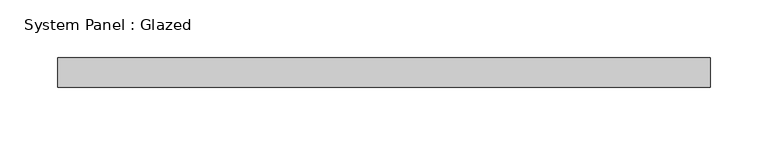
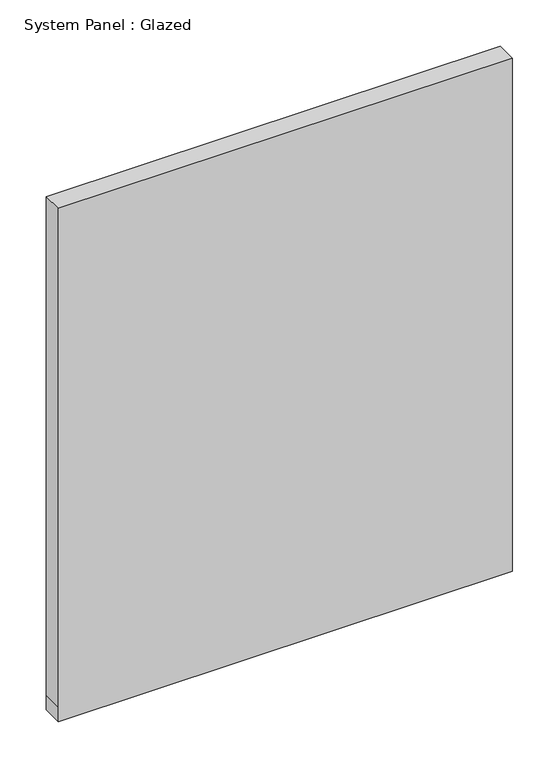
"""IFC4 building model written with IfcOpenShell, lengths in millimetres: plate geometry, System Panel : Glazed."""

from ifc_helpers import new_model, si_unit, frame, origin, place, context, project, spatial, polyline, outline, extrude, source, transform, mapped, element, save


def system_panel_glazed_6d48a8a8(model_context):
    return source(origin(), model_context, "Body", "SweptSolid", [
        extrude(outline(polyline([(0.0, -282.575), (0.0, 282.575), (19.05, 282.575), (675.1539078, 282.575), (675.1539078, -282.575), (19.05, -282.575), (0.0, -282.575)])), frame((0.0, 19.05, 0.0), z_axis=(0.0, 1.0, 0.0), x_axis=(0.0, 0.0, 1.0)), (0.0, 0.0, 1.0), 25.4),
    ])


if __name__ == "__main__":
    model = new_model("IFC4")
    model_context = context("Model", 3, world=origin())
    ifc_project = project(units=[si_unit("LENGTHUNIT", "METRE", prefix="MILLI")], contexts=[model_context])
    site = spatial("IfcSite", under=ifc_project)
    building = spatial("IfcBuilding", under=site)
    placement = place(None, origin())
    system_panel_glazed_shape = system_panel_glazed_6d48a8a8(model_context)
    element("IfcPlate", 1, ObjectType="System Panel : Glazed", at=placement, inside=building, context=model_context, shape_type="MappedRepresentation", body=[
        mapped(system_panel_glazed_shape, transform((0.0, 0.0, 0.0), x_axis=(1.0, 0.0, 0.0), y_axis=(0.0, 1.0, 0.0), z_axis=(0.0, 0.0, 1.0))),
    ])
    save(model, "model.ifc")

# Revit data of these elements
# Type "System Panel : Glazed"
#   Construction Type Id = "GSP4R"
#   Analytic Construction = "1/8 in Pilkington single glazing"
#   Visual Light Transmittance = 0.9
#   Solar Heat Gain Coefficient = 0.86
#   Heat Transfer Coefficient (U) = 1.18115 BTU/(h·ft²·°F)
#   Define Thermal Properties by = 1
# Element 1 (IfcPlate, "System Panel : Glazed")
#   Materials on its faces: "Glass"
# Materials
#   "Glass": class "Glass", colour RGB 0 128 192, transparency 0.75, Description = "Soda Lime Glass", Cost = 0
